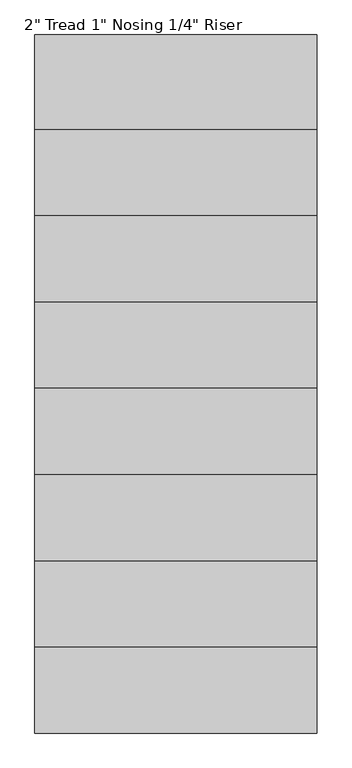
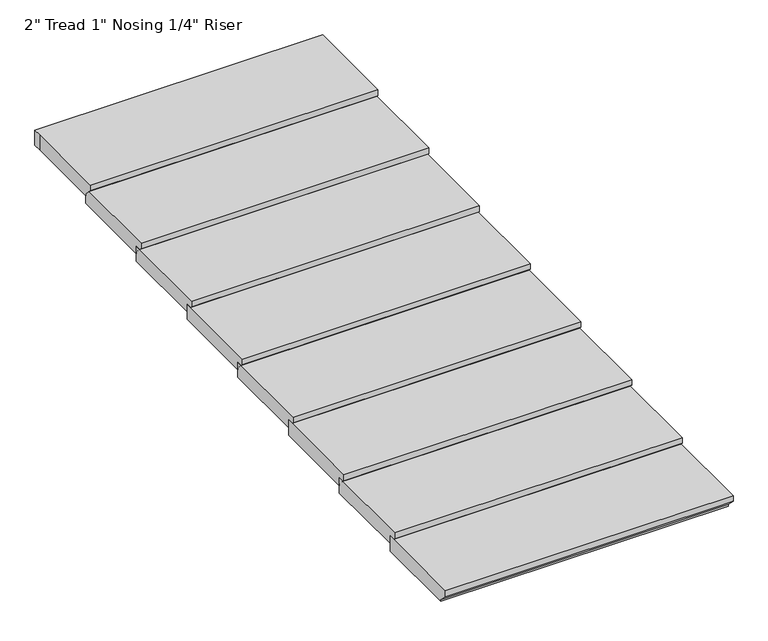
"""IFC4 building model written with IfcOpenShell, lengths in millimetres: stair flight geometry."""

from ifc_helpers import new_model, si_unit, origin, place, context, project, spatial, faceted_brep, source, transform, mapped, element, save


def stair_flight_42c3951d(model_context):
    return source(origin(), model_context, "Body", "Brep", [
        faceted_brep([(-6534.1867944, 11074.6230289, 3206.75), (-6534.1867944, 11074.6230289, 3225.8), (-7448.5867944, 11074.6230289, 3225.8), (-7448.5867944, 11074.6230289, 3206.75), (-6534.1867944, 11100.0230289, 3181.35), (-7448.5867944, 11100.0230289, 3181.35), (-6534.1867944, 11379.4230289, 3225.8), (-7448.5867944, 11379.4230289, 3225.8), (-7448.5867944, 11100.0230289, 3175.0), (-7448.5867944, 11379.4230289, 3175.0), (-6534.1867944, 11379.4230289, 3175.0), (-6534.1867944, 11100.0230289, 3175.0)], [[[0, 1, 2, 3]], [[4, 0, 3, 5]], [[2, 1, 6, 7]], [[8, 9, 10, 11]], [[2, 7, 9, 8, 5, 3]], [[8, 11, 4, 5]], [[6, 1, 0, 4, 11, 10]], [[7, 6, 10, 9]]]),
        faceted_brep([(-7448.5867944, 13335.2230289, 3403.6), (-7448.5867944, 13309.8230289, 3403.6), (-7448.5867944, 13030.4230289, 3403.6), (-6534.1867944, 13030.4230289, 3403.6), (-6534.1867944, 13335.2230289, 3403.6), (-7448.5867944, 13309.8230289, 3352.8), (-7448.5867944, 13335.2230289, 3352.8), (-6534.1867944, 13335.2230289, 3352.8), (-6534.1867944, 13055.8230289, 3352.8), (-7448.5867944, 13055.8230289, 3352.8), (-7448.5867944, 13055.8230289, 3359.15), (-7448.5867944, 13030.4230289, 3384.55), (-6534.1867944, 13055.8230289, 3359.15), (-6534.1867944, 13030.4230289, 3384.55)], [[[0, 1, 2, 3, 4]], [[5, 6, 7, 8, 9]], [[1, 0, 6, 5]], [[2, 1, 5, 9, 10, 11]], [[9, 8, 12, 10]], [[4, 3, 13, 12, 8, 7]], [[0, 4, 7, 6]], [[13, 3, 2, 11]], [[12, 13, 11, 10]]]),
        faceted_brep([(-7448.5867944, 11354.0230289, 3251.2), (-6534.1867944, 11354.0230289, 3251.2), (-6534.1867944, 11658.8230289, 3251.2), (-7448.5867944, 11658.8230289, 3251.2), (-7448.5867944, 11379.4230289, 3200.4), (-7448.5867944, 11658.8230289, 3200.4), (-6534.1867944, 11658.8230289, 3200.4), (-6534.1867944, 11379.4230289, 3200.4), (-7448.5867944, 11379.4230289, 3206.75), (-7448.5867944, 11354.0230289, 3232.15), (-6534.1867944, 11379.4230289, 3206.75), (-6534.1867944, 11354.0230289, 3232.15)], [[[0, 1, 2, 3]], [[4, 5, 6, 7]], [[0, 3, 5, 4, 8, 9]], [[4, 7, 10, 8]], [[2, 1, 11, 10, 7, 6]], [[3, 2, 6, 5]], [[11, 1, 0, 9]], [[10, 11, 9, 8]]]),
        faceted_brep([(-7448.5867944, 11633.4230289, 3276.6), (-6534.1867944, 11633.4230289, 3276.6), (-6534.1867944, 11938.2230289, 3276.6), (-7448.5867944, 11938.2230289, 3276.6), (-7448.5867944, 11658.8230289, 3225.8), (-7448.5867944, 11938.2230289, 3225.8), (-6534.1867944, 11938.2230289, 3225.8), (-6534.1867944, 11658.8230289, 3225.8), (-7448.5867944, 11658.8230289, 3232.15), (-7448.5867944, 11633.4230289, 3257.55), (-6534.1867944, 11658.8230289, 3232.15), (-6534.1867944, 11633.4230289, 3257.55)], [[[0, 1, 2, 3]], [[4, 5, 6, 7]], [[0, 3, 5, 4, 8, 9]], [[4, 7, 10, 8]], [[2, 1, 11, 10, 7, 6]], [[3, 2, 6, 5]], [[11, 1, 0, 9]], [[10, 11, 9, 8]]]),
        faceted_brep([(-7448.5867944, 11912.8230289, 3302.0), (-6534.1867944, 11912.8230289, 3302.0), (-6534.1867944, 12217.6230289, 3302.0), (-7448.5867944, 12217.6230289, 3302.0), (-7448.5867944, 11938.2230289, 3251.2), (-7448.5867944, 12217.6230289, 3251.2), (-6534.1867944, 12217.6230289, 3251.2), (-6534.1867944, 11938.2230289, 3251.2), (-7448.5867944, 11938.2230289, 3257.55), (-7448.5867944, 11912.8230289, 3282.95), (-6534.1867944, 11938.2230289, 3257.55), (-6534.1867944, 11912.8230289, 3282.95)], [[[0, 1, 2, 3]], [[4, 5, 6, 7]], [[0, 3, 5, 4, 8, 9]], [[4, 7, 10, 8]], [[2, 1, 11, 10, 7, 6]], [[3, 2, 6, 5]], [[11, 1, 0, 9]], [[10, 11, 9, 8]]]),
        faceted_brep([(-7448.5867944, 12192.2230289, 3327.4), (-6534.1867944, 12192.2230289, 3327.4), (-6534.1867944, 12497.0230289, 3327.4), (-7448.5867944, 12497.0230289, 3327.4), (-7448.5867944, 12217.6230289, 3276.6), (-7448.5867944, 12497.0230289, 3276.6), (-6534.1867944, 12497.0230289, 3276.6), (-6534.1867944, 12217.6230289, 3276.6), (-7448.5867944, 12217.6230289, 3282.95), (-7448.5867944, 12192.2230289, 3308.35), (-6534.1867944, 12217.6230289, 3282.95), (-6534.1867944, 12192.2230289, 3308.35)], [[[0, 1, 2, 3]], [[4, 5, 6, 7]], [[0, 3, 5, 4, 8, 9]], [[4, 7, 10, 8]], [[2, 1, 11, 10, 7, 6]], [[3, 2, 6, 5]], [[11, 1, 0, 9]], [[10, 11, 9, 8]]]),
        faceted_brep([(-7448.5867944, 12471.6230289, 3352.8), (-6534.1867944, 12471.6230289, 3352.8), (-6534.1867944, 12776.4230289, 3352.8), (-7448.5867944, 12776.4230289, 3352.8), (-7448.5867944, 12497.0230289, 3302.0), (-7448.5867944, 12776.4230289, 3302.0), (-6534.1867944, 12776.4230289, 3302.0), (-6534.1867944, 12497.0230289, 3302.0), (-7448.5867944, 12497.0230289, 3308.35), (-7448.5867944, 12471.6230289, 3333.75), (-6534.1867944, 12497.0230289, 3308.35), (-6534.1867944, 12471.6230289, 3333.75)], [[[0, 1, 2, 3]], [[4, 5, 6, 7]], [[0, 3, 5, 4, 8, 9]], [[4, 7, 10, 8]], [[2, 1, 11, 10, 7, 6]], [[3, 2, 6, 5]], [[11, 1, 0, 9]], [[10, 11, 9, 8]]]),
        faceted_brep([(-7448.5867944, 12751.0230289, 3378.2), (-6534.1867944, 12751.0230289, 3378.2), (-6534.1867944, 13055.8230289, 3378.2), (-7448.5867944, 13055.8230289, 3378.2), (-7448.5867944, 12776.4230289, 3327.4), (-7448.5867944, 13055.8230289, 3327.4), (-6534.1867944, 13055.8230289, 3327.4), (-6534.1867944, 12776.4230289, 3327.4), (-7448.5867944, 12776.4230289, 3333.75), (-7448.5867944, 12751.0230289, 3359.15), (-6534.1867944, 12776.4230289, 3333.75), (-6534.1867944, 12751.0230289, 3359.15)], [[[0, 1, 2, 3]], [[4, 5, 6, 7]], [[0, 3, 5, 4, 8, 9]], [[4, 7, 10, 8]], [[2, 1, 11, 10, 7, 6]], [[3, 2, 6, 5]], [[11, 1, 0, 9]], [[10, 11, 9, 8]]]),
    ])


if __name__ == "__main__":
    model = new_model("IFC4")
    model_context = context("Model", 3, world=origin())
    ifc_project = project(units=[si_unit("LENGTHUNIT", "METRE", prefix="MILLI")], contexts=[model_context])
    site = spatial("IfcSite", under=ifc_project)
    building = spatial("IfcBuilding", under=site)
    placement = place(None, origin())
    stair_flight_shape = stair_flight_42c3951d(model_context)
    element("IfcStairFlight", 1, ObjectType="2\" Tread 1\" Nosing 1/4\" Riser", at=placement, inside=building, context=model_context, shape_type="MappedRepresentation", body=[
        mapped(stair_flight_shape, transform((0.0, 0.0, 0.0), x_axis=(1.0, 0.0, 0.0), y_axis=(0.0, 1.0, 0.0), z_axis=(0.0, 0.0, 1.0))),
    ])
    save(model, "model.ifc")
